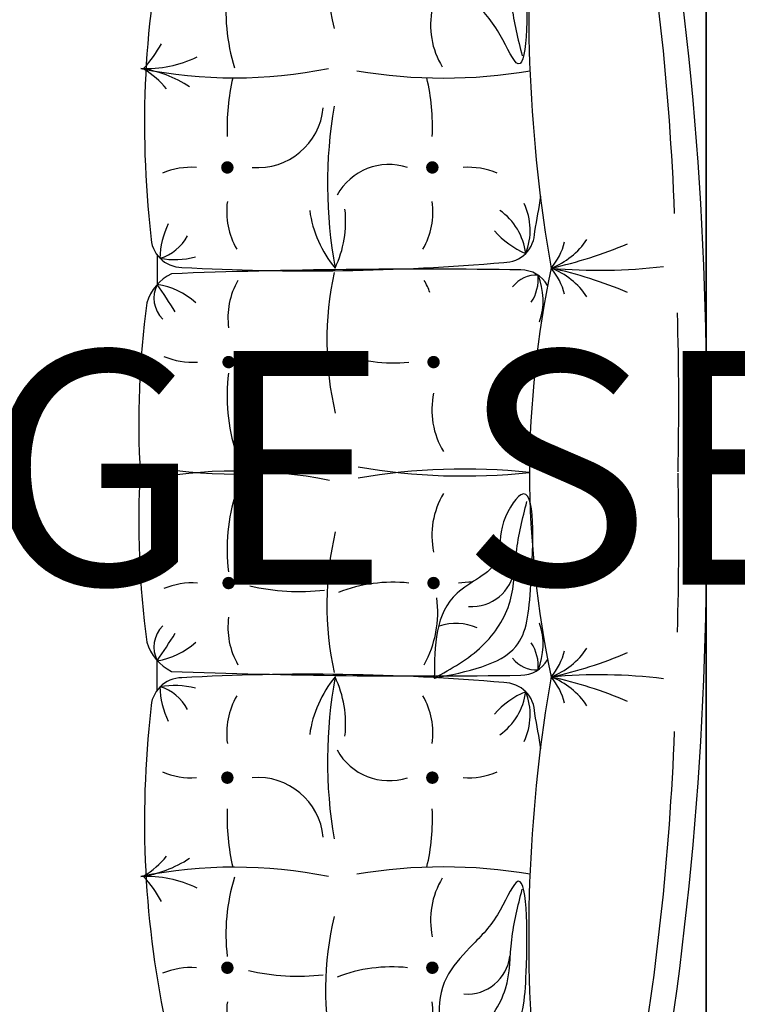
# Model space of a CAD drawing. Units: inches. Extents: x 844 to 2234, y 346 to 1084.
# Tile 87 of 93: x 2012 to 2031, y 688 to 713. Entities that reach past the tile are written whole.
import ezdxf

# ---------------------------------------------------------------- set-up
doc = ezdxf.new("R2010")
doc.units = ezdxf.units.IN
doc.header["$MEASUREMENT"] = 0
for name, color, linetype, lineweight in [('A-ANNO-DIMS', 2, 'Continuous', 18), ('A-WALL', 7, 'Continuous', 35), ('furniture', 8, 'Continuous', 18)]:
    doc.layers.add(name, color=color, linetype=linetype, lineweight=lineweight)
doc.layers.add('RA-AP-01$0$FURN', color=3, linetype='Continuous')
doc.layers.add('RA-AP-01$0$WOOD', color=64, linetype='Continuous')
doc.styles.get("Standard").update_dxf_attribs({"font": 'arial.ttf'})
doc.dimstyles.get("Standard").update_dxf_attribs({"dimtxt": 6, "dimasz": 3, "dimexe": 0.18, "dimexo": 0.0625, "dimgap": 0.09, "dimtad": 0, "dimtih": 1, "dimtoh": 1, "dimdec": 1, "dimzin": 0, "dimdsep": 46, "dimlunit": 3, "dimtxsty": 'Standard', "dimblk": 'ARCHTICK', "dimcen": 0.09, "dimadec": 0, "dimazin": 0, "dimtfac": 1, "dimtdec": 1, "dimtofl": 0, "dimtmove": 0, "dimatfit": 3, "dimfxl": 1, "dimtolj": 1, "dimtzin": 0, "dimarcsym": 0})

# ---------------------------------------------------------------- blocks, each defined once
blk = doc.blocks.new('A$C7EE91E48')
at = {"layer": 'RA-AP-01$0$FURN'}
for p, q in [((8.4752, -8.8836), (8.5044, -8.8836)), ((8.5044, -8.8836), (8.5227, -8.8836)), ((9.1476, -8.8836), (9.1292, -8.8836)), ((9.1768, -8.8836), (9.1476, -8.8836))]:
    blk.add_line(p, q, dxfattribs=at)
at = {"layer": 'RA-AP-01$0$FURN', "const_width": 0.01}
for points in [[(8.0279, -9.0019, -1), (8.0279, -8.9919, -1)], [(8.3342, -9.0019, 1), (8.3342, -8.9919, 1)], [(8.6479, -9.0039, -1), (8.6479, -8.9939, -1)], [(9.004, -9.0039, 1), (9.004, -8.9939, 1)], [(9.3177, -9.0019, -1), (9.3177, -8.9919, -1)], [(8.0279, -9.3223, 1), (8.0279, -9.3323, 1)], [(8.3342, -9.3223, -1), (8.3342, -9.3323, -1)], [(8.6479, -9.3243, 1), (8.6479, -9.3343, 1)], [(9.004, -9.3243, -1), (9.004, -9.3343, -1)], [(9.3177, -9.3223, 1), (9.3177, -9.3323, 1)]]:
    blk.add_lwpolyline(points, format="xyb", close=True, dxfattribs=at)
at = {"layer": 'RA-AP-01$0$FURN'}
for centre, radius, start, end in [((8.744, -10.2748), 1.4207, 86.5948, 97.7424), ((8.9079, -10.2748), 1.4207, 82.2576, 93.4052), ((8.2641, -10.4424), 1.5791, 83.4116, 102.408), ((8.0633, -8.7497), 0.1579, 296.9155, 314.5948), ((7.9834, -8.8653), 0.1916, 334.4169, 2.4147), ((7.4244, -9.0082), 0.7655, 348.5826, 11.3727), ((8.3595, -8.8326), 0.1864, 187.6182, 213.7074), ((8.3098, -8.7788), 0.1579, 211.9342, 229.6135), ((8.5734, -8.9396), 0.0754, 106.0166, 154.1254), ((8.0629, -9.0102), 0.7655, 348.5826, 11.3727), ((9.589, -9.0102), 0.7655, 168.6273, 191.4174), ((9.0785, -8.9396), 0.0754, 25.8746, 73.9834), ((9.3879, -10.4424), 1.5791, 77.592, 96.5884), ((9.3421, -8.7788), 0.1579, 310.3865, 328.0658), ((9.2924, -8.8326), 0.1864, 326.2926, 352.3818), ((10.2276, -9.0082), 0.7655, 168.6273, 191.4174), ((9.6686, -8.8653), 0.1916, 177.5853, 205.5831), ((9.5886, -8.7497), 0.1579, 225.4052, 243.0845), ((8.4452, -8.9237), 0.05, 0, 90), ((8.5446, -8.9264), 0.0479, 44.5975, 117.1929), ((8.6431, -8.8646), 0.1219, 188.9538, 221.9624), ((9.1542, -7.9707), 1.1102, 235.3335, 238.0671), ((9.1073, -8.9264), 0.0479, 62.8071, 135.4025), ((8.4977, -7.9707), 1.1102, 301.9329, 304.6665), ((9.0089, -8.8646), 0.1219, 318.0376, 351.0462), ((9.2067, -8.9237), 0.05, 90, 180), ((7.9069, -8.939), 0.1213, 356.2685, 22.6624), ((8.4553, -8.939), 0.1213, 157.3376, 183.7315), ((8.4834, -9.0206), 0.1324, 91.1993, 116.1112), ((8.411, -8.8679), 0.0726, 297.3225, 343.6441), ((8.3504, -8.912), 0.1324, 345.3922, 10.3041), ((8.5269, -8.941), 0.1213, 356.2685, 22.6624), ((9.1251, -8.941), 0.1213, 157.3376, 183.7315), ((9.3016, -8.912), 0.1324, 169.6959, 194.6078), ((9.1686, -9.0206), 0.1324, 63.8888, 88.8007), ((9.241, -8.8679), 0.0726, 196.3559, 242.6775), ((9.1967, -8.939), 0.1213, 356.2685, 22.6624), ((19.2274, -9.306), 10.7293, 177.86728, 180.87576), ((-1.5755, -9.306), 10.7293, 359.12424, 2.13272), ((4.8029, -9.1271), 3.698, 355.1082, 3.1536), ((12.8491, -9.1271), 3.698, 176.8464, 184.8918), ((7.9567, -9.1172), 0.1214, 82.3083, 119.8581), ((8.0823, -9.2969), 0.3024, 72.4119, 96.9055), ((8.2692, -9.3452), 0.3487, 87.5342, 103.1608), ((8.4055, -9.1172), 0.1214, 60.1419, 97.6917), ((8.5767, -9.1192), 0.1214, 82.3083, 119.8581), ((8.7023, -9.299), 0.3024, 72.4119, 96.9055), ((8.9496, -9.299), 0.3024, 83.0945, 107.5881), ((9.0753, -9.1192), 0.1214, 60.1419, 97.6917), ((9.2465, -9.1172), 0.1214, 82.3083, 119.8581), ((9.3827, -9.3452), 0.3487, 76.8392, 92.4658), ((9.5696, -9.2969), 0.3024, 83.0945, 107.5881), ((8.3659, -9.111), 0.3517, 166.8325, 186.5875), ((8.2285, -9.0458), 0.106, 275.1859, 4.8073), ((8.9859, -9.113), 0.3517, 166.8325, 186.5875), ((8.666, -9.113), 0.3517, 353.4125, 13.1675), ((9.4234, -9.0458), 0.106, 175.1927, 264.8141), ((8.378, -9.3133), 0.1855, 50.3168, 82.0523), ((9.2739, -9.3133), 0.1855, 97.9477, 129.6832), ((7.9929, -9.6653), 0.5101, 76.6878, 102.3818), ((9.6591, -9.6653), 0.5101, 77.6182, 103.3122), ((8.3614, -9.9068), 0.7485, 79.6011, 99.6906), ((8.4207, -9.0107), 0.1769, 263.6796, 295.3608), ((8.6129, -9.6673), 0.5101, 76.6878, 102.3818), ((9.0391, -9.6673), 0.5101, 77.6182, 103.3122), ((9.2906, -9.9068), 0.7485, 80.3094, 100.3989), ((9.2312, -9.0107), 0.1769, 244.6392, 276.3204), ((7.785, -9.2618), 0.2442, 354.0076, 21.0983), ((8.4248, -9.2574), 0.0954, 118.8034, 198.2253), ((8.405, -9.2638), 0.2442, 354.0076, 21.0983), ((9.2469, -9.2638), 0.2442, 158.9017, 185.9924), ((9.2271, -9.2574), 0.0954, 341.7747, 61.1966), ((7.367, -9.3453), 0.8233, 350.2449, 9.7551), ((7.8327, -9.3782), 0.9989, 353.9343, 9.823), ((9.8193, -9.3782), 0.9989, 170.177, 186.0657), ((10.285, -9.3453), 0.8233, 170.2449, 189.7551), ((7.9567, -9.2069), 0.1214, 240.1419, 277.6917), ((8.4055, -9.2069), 0.1214, 262.3083, 299.8581), ((8.6002, -9.1634), 0.1726, 240.9024, 278.0073), ((9.0753, -9.209), 0.1214, 289.6086, 299.8581), ((9.2465, -9.2069), 0.1214, 240.1419, 277.6917), ((8.1048, -9.4539), 0.1295, 58.6204, 102.0099), ((8.2692, -8.9789), 0.3487, 256.8392, 272.4658), ((8.7248, -9.456), 0.1295, 58.6204, 102.0099), ((8.9271, -9.456), 0.1295, 77.9901, 121.3796), ((9.3827, -8.9789), 0.3487, 267.5342, 283.1608), ((9.5471, -9.4539), 0.1295, 77.9901, 121.3796), ((8.5004, -9.3657), 0.0825, 335.8161, 19.2747), ((8.0543, -9.3837), 0.0689, 175.5384, 263.5805), ((8.4553, -9.3851), 0.1213, 176.2685, 202.6624), ((8.405, -9.3948), 0.2442, 0.7304, 5.9924), ((9.1967, -9.3851), 0.1213, 337.3376, 3.7315), ((8.6789, -9.3912), 0.0689, 175.5384, 263.5805), ((8.4847, -9.3794), 0.0991, 214.8912, 263.0774), ((8.3451, -9.5317), 0.1386, 22.9132, 48.7711), ((9.3068, -9.5317), 0.1386, 131.2289, 157.0868), ((9.1673, -9.3794), 0.0991, 276.9226, 325.1088), ((8.4374, -9.4424), 0.05, 270, 0), ((8.5556, -9.4948), 0.0479, 127.3166, 183.4247), ((9.0963, -9.4948), 0.0479, 356.5753, 52.6834), ((9.2146, -9.4424), 0.05, 180, 270), ((8.5494, -9.4699), 0.05, 180, 239.8522), ((9.1025, -9.4699), 0.05, 300.1478, 360), ((8.0772, -11.9348), 2.4522, 80.1542, 94.8039), ((8.4354, -9.3857), 0.0993, 244.3656, 292.0953), ((8.8331, -11.1187), 1.6349, 90.2483, 101.88), ((8.514, -9.4297), 0.0683, 264.7816, 303.327), ((8.8189, -11.1187), 1.6349, 78.12, 89.7517), ((9.1379, -9.4297), 0.0683, 236.673, 275.2184), ((9.5748, -11.9348), 2.4522, 85.1961, 99.8458), ((9.2166, -9.3857), 0.0993, 247.9047, 295.6344), ((8.1811, -8.1864), 1.3309, 278.6229, 281.1036), ((8.5483, -9.4017), 0.1042, 247.1307, 289.5172), ((9.1036, -9.4017), 0.1042, 250.4828, 292.8693), ((9.4709, -8.1864), 1.3309, 258.8964, 261.3771), ((8.3825, -9.4751), 0.122, 303.7136, 339.041), ((8.4279, -9.4377), 0.1062, 284.3648, 310.2303), ((7.8141, -9.3689), 0.6986, 337.0091, 347.612), ((7.6413, -9.5958), 0.8587, 353.0376, 5.1445), ((8.6105, -9.4751), 0.122, 200.959, 236.2864), ((8.5651, -9.4377), 0.1062, 229.7697, 255.6352), ((9.1788, -9.3689), 0.6986, 192.388, 202.9909), ((9.0415, -9.4751), 0.122, 303.7136, 339.041), ((9.0869, -9.4377), 0.1062, 284.3648, 310.2303), ((8.4731, -9.3689), 0.6986, 337.0091, 347.612), ((10.0107, -9.5958), 0.8587, 174.8555, 186.9624), ((9.2694, -9.4751), 0.122, 200.959, 236.2864), ((9.224, -9.4377), 0.1062, 229.7697, 255.6352), ((9.8378, -9.3689), 0.6986, 192.388, 202.9909), ((8.5724, -5.4361), 4.2848, 259.7801, 267.8084), ((9.0796, -5.4361), 4.2848, 272.1916, 280.2199), ((8.7159, -4.2841), 5.4854, 259.9939, 271.1496), ((8.936, -4.2841), 5.4854, 268.8504, 280.0061), ((8.7159, -4.2841), 5.4404, 268.4485, 271.1496), ((8.936, -4.2841), 5.4404, 268.8504, 271.5515)]:
    blk.add_arc(centre, radius, start, end, dxfattribs=at)
for points, knots in [([(7.8747, -9.3485), (7.9231, -9.3393), (7.9933, -9.326), (8.0638, -9.3901), (8.1031, -9.4315), (8.221, -9.4812), (8.0194, -9.4811), (7.9064, -9.4702), (7.8857, -9.3906), (7.8747, -9.3485)], [0, 0, 0, 0, 0.1367587, 0.1981302, 0.267773, 0.3281195, 0.4737578, 0.5765194, 0.6920332, 0.6920332, 0.6920332, 0.6920332]), ([(8.4947, -9.3305), (8.5098, -9.3579), (8.5387, -9.4102), (8.6151, -9.4603), (8.6994, -9.4595), (8.7521, -9.4728), (8.7791, -9.4797)], [0, 0, 0, 0, 0.0929945, 0.178054, 0.2574251, 0.3407808, 0.3407808, 0.3407808, 0.3407808]), ([(8.4947, -9.3305), (8.547, -9.3311), (8.63, -9.3319), (8.67, -9.4425), (8.7389, -9.4316), (8.8424, -9.4963), (8.6448, -9.4874), (8.5233, -9.4759), (8.5051, -9.3838), (8.4947, -9.3305)], [0, 0, 0, 0, 0.1415752, 0.2249019, 0.2789443, 0.3392908, 0.4849291, 0.5876907, 0.7285367, 0.7285367, 0.7285367, 0.7285367]), ([(9.7773, -9.3485), (9.7288, -9.3393), (9.6586, -9.326), (9.5882, -9.3901), (9.5488, -9.4315), (9.4309, -9.4812), (9.6325, -9.4811), (9.7455, -9.4702), (9.7663, -9.3906), (9.7773, -9.3485)], [0, 0, 0, 0, 0.1367587, 0.1981302, 0.267773, 0.3281195, 0.4737578, 0.5765194, 0.6920332, 0.6920332, 0.6920332, 0.6920332]), ([(7.8747, -9.3485), (7.8896, -9.3663), (7.9228, -9.4056), (7.9899, -9.4532), (8.0749, -9.4519), (8.1275, -9.4653), (8.1544, -9.4722)], [0, 0, 0, 0, 0.0700185, 0.155078, 0.2344492, 0.3178049, 0.3178049, 0.3178049, 0.3178049]), ([(9.7773, -9.3485), (9.7623, -9.3663), (9.7292, -9.4056), (9.662, -9.4532), (9.577, -9.4519), (9.5245, -9.4653), (9.4975, -9.4722)], [0, 0, 0, 0, 0.0700185, 0.155078, 0.2344492, 0.3178049, 0.3178049, 0.3178049, 0.3178049])]:
    blk.add_open_spline(points, degree=3, knots=knots, dxfattribs=at)
blk = doc.blocks.new('A$C5D2F253E')
at = {"layer": 'RA-AP-01$0$WOOD', "xscale": -1, "rotation": 180}
blk.add_blockref('A$C7EE91E48', (-8.833, -7.2888), dxfattribs=at)
blk = doc.blocks.new('_ArchTick')
at = {"color": 0, "linetype": 'ByBlock', "const_width": 0.15}
blk.add_lwpolyline([(-0.5, -0.5), (0.5, 0.5)], dxfattribs=at)
blk = doc.blocks.new('*D121')
at = {"layer": 'A-ANNO-DIMS', "color": 0, "lineweight": -2, "transparency": 16777216}
for p, q in [((2030.272, 734.263), (2040.245, 734.263)), ((2040.065, 734.263), (2040.065, 704.604)), ((2040.065, 668.557), (2040.065, 698.216)), ((2030.272, 668.557), (2040.245, 668.557))]:
    blk.add_line(p, q, dxfattribs=at)
at = {"layer": 'Defpoints', "color": 0, "transparency": 16777216}
for p in [(2030.209, 734.263), (2040.065, 734.263), (2030.209, 668.557)]:
    blk.add_point(p, dxfattribs=at)
at = {"layer": 'A-ANNO-DIMS', "color": 0, "lineweight": -2, "transparency": 16777216, "xscale": 3, "yscale": 3, "zscale": 3}
for p, rotation in [((2040.065, 734.263), 90), ((2040.065, 668.557), 270)]:
    blk.add_blockref('_ArchTick', p, dxfattribs=dict(at, rotation=rotation))
at = {"layer": 'A-ANNO-DIMS', "color": 0, "transparency": 16777216, "insert": (2040.065, 701.41), "char_height": 6, "attachment_point": 5}
blk.add_mtext('\\A1;LOUNGE SET 5\'-5 1/2" TYP.', dxfattribs=at)

msp = doc.modelspace()

# ---------------------------------------------------------------- linework, layer by layer
at = {"layer": 'A-WALL'}
msp.add_line((2030.099, 766.455), (2030.099, 629.455), dxfattribs=at)

# ---------------------------------------------------------------- block references
at = {"layer": 'furniture', "xscale": -15.94108302203742, "yscale": 15.94108302203742, "zscale": 15.94108302203742, "rotation": 270}
msp.add_blockref('A$C5D2F253E', (1990.567, 701.403), dxfattribs=at)

# ---------------------------------------------------------------- dimensions: what is measured, and where the dimension line sits
at = {"layer": 'A-ANNO-DIMS'}
dim = msp.add_linear_dim(base=(2040.065, 734.263), p1=(2030.209, 668.557), p2=(2030.209, 734.263), angle=90, text='LOUNGE SET <> TYP.', dimstyle='Standard', override={"dimdec": 1, "dimlfac": 1, "dimrnd": 0, "dimzin": 1, "dimdsep": 46, "dimlunit": 4, "dimfrac": 2}, dxfattribs=at)
dim.commit()
dim.dimension.update_dxf_attribs({"geometry": '*D121', "text_midpoint": (2040.065, 701.41)})

doc.saveas('drawing.dxf')
